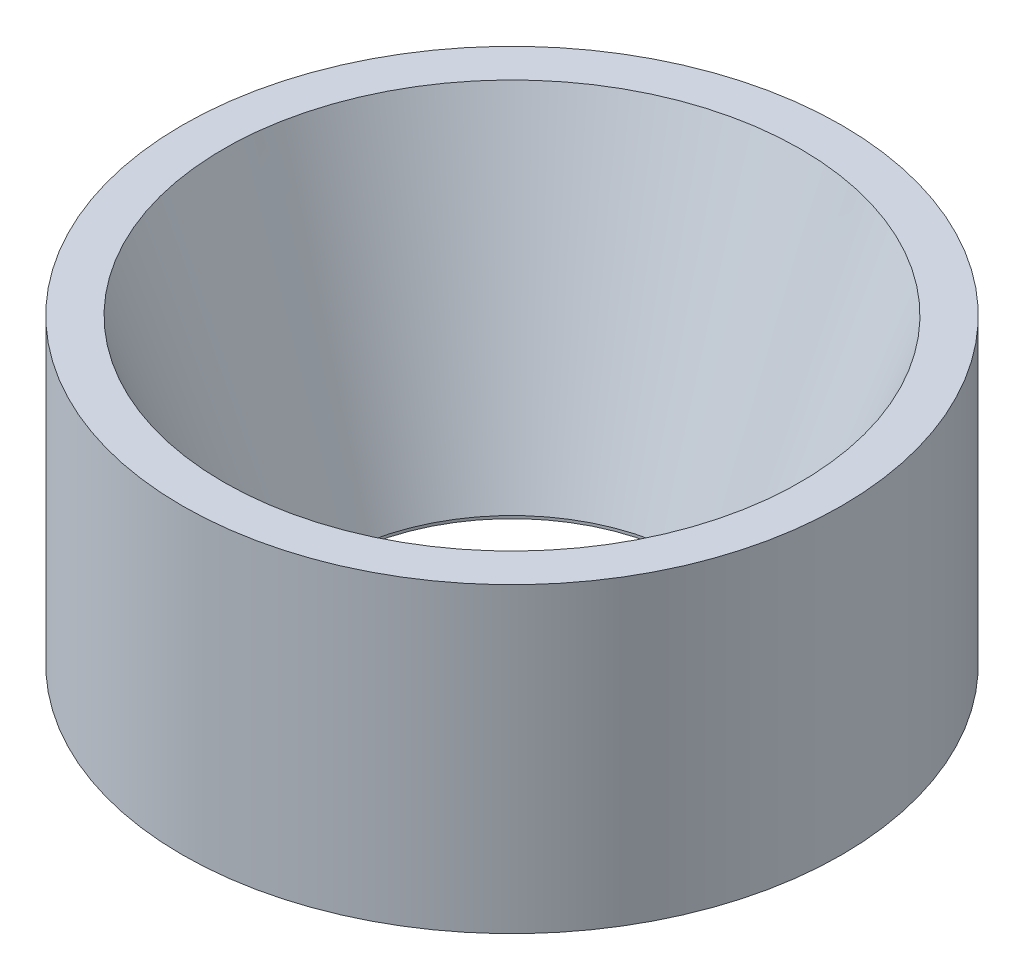
ISO-10303-21;
HEADER;
FILE_DESCRIPTION(('STEP AP214'),'2;1');
FILE_NAME('part.step','',(''),(''),'','','');
FILE_SCHEMA(('AUTOMOTIVE_DESIGN { 1 0 10303 214 1 1 1 1 }'));
ENDSEC;
DATA;
#1=APPLICATION_CONTEXT('core data for automotive mechanical design processes');
#2=APPLICATION_PROTOCOL_DEFINITION('international standard','automotive_design',2000,#1);
#3=PRODUCT_CONTEXT('',#1,'mechanical');
#4=PRODUCT('Part','Part','',(#3));
#5=PRODUCT_RELATED_PRODUCT_CATEGORY('part','',(#4));
#6=PRODUCT_DEFINITION_FORMATION('','',#4);
#7=PRODUCT_DEFINITION_CONTEXT('part definition',#1,'design');
#8=PRODUCT_DEFINITION('design','',#6,#7);
#9=PRODUCT_DEFINITION_SHAPE('','',#8);
#10=(LENGTH_UNIT() NAMED_UNIT(*) SI_UNIT(.MILLI.,.METRE.));
#11=(NAMED_UNIT(*) PLANE_ANGLE_UNIT() SI_UNIT($,.RADIAN.));
#12=(NAMED_UNIT(*) SI_UNIT($,.STERADIAN.) SOLID_ANGLE_UNIT());
#13=UNCERTAINTY_MEASURE_WITH_UNIT(LENGTH_MEASURE(1.E-05),#10,'distance_accuracy_value','');
#14=(GEOMETRIC_REPRESENTATION_CONTEXT(3) GLOBAL_UNCERTAINTY_ASSIGNED_CONTEXT((#13)) GLOBAL_UNIT_ASSIGNED_CONTEXT((#10,
#11,#12)) REPRESENTATION_CONTEXT('',''));
#15=CARTESIAN_POINT('',(0.,0.,0.));
#16=DIRECTION('',(0.,0.,1.));
#17=DIRECTION('',(1.,0.,0.));
#18=AXIS2_PLACEMENT_3D('',#15,#16,#17);
#19=CARTESIAN_POINT('',(0.,22.,0.));
#20=DIRECTION('',(0.,-1.,0.));
#21=DIRECTION('',(0.,0.,-1.));
#22=AXIS2_PLACEMENT_3D('',#19,#20,#21);
#23=CYLINDRICAL_SURFACE('',#22,24.);
#24=CARTESIAN_POINT('',(0.,22.,0.));
#25=DIRECTION('',(0.,1.,0.));
#26=DIRECTION('',(0.,0.,1.));
#27=AXIS2_PLACEMENT_3D('',#24,#25,#26);
#28=CIRCLE('',#27,24.);
#29=CARTESIAN_POINT('',(0.,22.,24.));
#30=VERTEX_POINT('',#29);
#31=EDGE_CURVE('E11',#30,#30,#28,.T.);
#32=ORIENTED_EDGE('',*,*,#31,.F.);
#33=EDGE_LOOP('',(#32));
#34=FACE_BOUND('',#33,.T.);
#35=CARTESIAN_POINT('',(0.,0.,0.));
#36=DIRECTION('',(0.,1.,0.));
#37=DIRECTION('',(0.,0.,1.));
#38=AXIS2_PLACEMENT_3D('',#35,#36,#37);
#39=CIRCLE('',#38,24.);
#40=CARTESIAN_POINT('',(0.,0.,24.));
#41=VERTEX_POINT('',#40);
#42=EDGE_CURVE('E48',#41,#41,#39,.T.);
#43=ORIENTED_EDGE('',*,*,#42,.T.);
#44=EDGE_LOOP('',(#43));
#45=FACE_BOUND('',#44,.T.);
#46=ADVANCED_FACE('F39',(#34,#45),#23,.T.);
#47=CARTESIAN_POINT('',(0.,22.,0.));
#48=DIRECTION('',(0.,1.,0.));
#49=DIRECTION('',(0.,0.,1.));
#50=AXIS2_PLACEMENT_3D('',#47,#48,#49);
#51=PLANE('',#50);
#52=CARTESIAN_POINT('',(0.,22.,0.));
#53=DIRECTION('',(0.,1.,0.));
#54=DIRECTION('',(0.,0.,1.));
#55=AXIS2_PLACEMENT_3D('',#52,#53,#54);
#56=CIRCLE('',#55,21.);
#57=CARTESIAN_POINT('',(0.,22.,21.));
#58=VERTEX_POINT('',#57);
#59=EDGE_CURVE('E52',#58,#58,#56,.T.);
#60=ORIENTED_EDGE('',*,*,#59,.F.);
#61=EDGE_LOOP('',(#60));
#62=FACE_BOUND('',#61,.T.);
#63=ORIENTED_EDGE('',*,*,#31,.T.);
#64=EDGE_LOOP('',(#63));
#65=FACE_BOUND('',#64,.T.);
#66=ADVANCED_FACE('F81',(#62,#65),#51,.T.);
#67=CARTESIAN_POINT('',(0.,0.,0.));
#68=DIRECTION('',(0.,1.,0.));
#69=DIRECTION('',(0.,0.,1.));
#70=AXIS2_PLACEMENT_3D('',#67,#68,#69);
#71=PLANE('',#70);
#72=CARTESIAN_POINT('',(0.,0.,0.));
#73=DIRECTION('',(0.,1.,0.));
#74=DIRECTION('',(0.,0.,1.));
#75=AXIS2_PLACEMENT_3D('',#72,#73,#74);
#76=CIRCLE('',#75,13.);
#77=CARTESIAN_POINT('',(0.,0.,13.));
#78=VERTEX_POINT('',#77);
#79=EDGE_CURVE('E61',#78,#78,#76,.F.);
#80=ORIENTED_EDGE('',*,*,#79,.F.);
#81=EDGE_LOOP('',(#80));
#82=FACE_BOUND('',#81,.T.);
#83=ORIENTED_EDGE('',*,*,#42,.F.);
#84=EDGE_LOOP('',(#83));
#85=FACE_BOUND('',#84,.T.);
#86=ADVANCED_FACE('F85',(#82,#85),#71,.F.);
#87=CARTESIAN_POINT('',(0.,0.199999999999999,0.));
#88=DIRECTION('',(0.,1.,0.));
#89=DIRECTION('',(0.,0.,1.));
#90=AXIS2_PLACEMENT_3D('',#87,#88,#89);
#91=CONICAL_SURFACE('',#90,13.,0.351714335776);
#92=ORIENTED_EDGE('',*,*,#59,.T.);
#93=EDGE_LOOP('',(#92));
#94=FACE_BOUND('',#93,.T.);
#95=CARTESIAN_POINT('',(0.,0.199999999999999,0.));
#96=DIRECTION('',(0.,1.,0.));
#97=DIRECTION('',(0.,0.,1.));
#98=AXIS2_PLACEMENT_3D('',#95,#96,#97);
#99=CIRCLE('',#98,13.);
#100=CARTESIAN_POINT('',(0.,0.199999999999999,13.));
#101=VERTEX_POINT('',#100);
#102=EDGE_CURVE('E58',#101,#101,#99,.T.);
#103=ORIENTED_EDGE('',*,*,#102,.F.);
#104=EDGE_LOOP('',(#103));
#105=FACE_BOUND('',#104,.T.);
#106=ADVANCED_FACE('F71',(#94,#105),#91,.F.);
#107=CARTESIAN_POINT('',(0.,-0.000999999999999997,0.));
#108=DIRECTION('',(0.,1.,0.));
#109=DIRECTION('',(0.,0.,1.));
#110=AXIS2_PLACEMENT_3D('',#107,#108,#109);
#111=CYLINDRICAL_SURFACE('',#110,13.);
#112=ORIENTED_EDGE('',*,*,#102,.T.);
#113=EDGE_LOOP('',(#112));
#114=FACE_BOUND('',#113,.T.);
#115=ORIENTED_EDGE('',*,*,#79,.T.);
#116=EDGE_LOOP('',(#115));
#117=FACE_BOUND('',#116,.T.);
#118=ADVANCED_FACE('F63',(#114,#117),#111,.F.);
#119=CLOSED_SHELL('',(#46,#66,#86,#106,#118));
#120=MANIFOLD_SOLID_BREP('B2',#119);
#121=ADVANCED_BREP_SHAPE_REPRESENTATION('',(#18,#120),#14);
#122=SHAPE_DEFINITION_REPRESENTATION(#9,#121);
ENDSEC;
END-ISO-10303-21;
